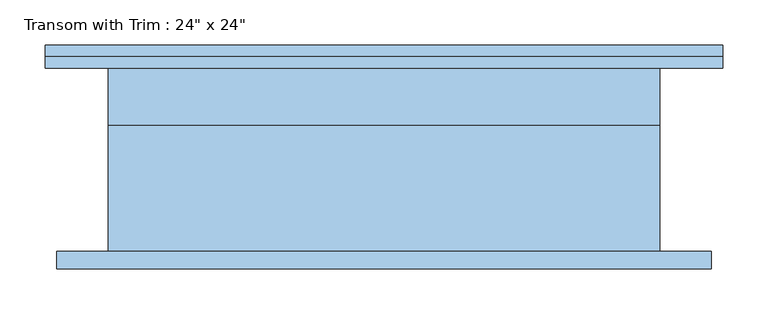
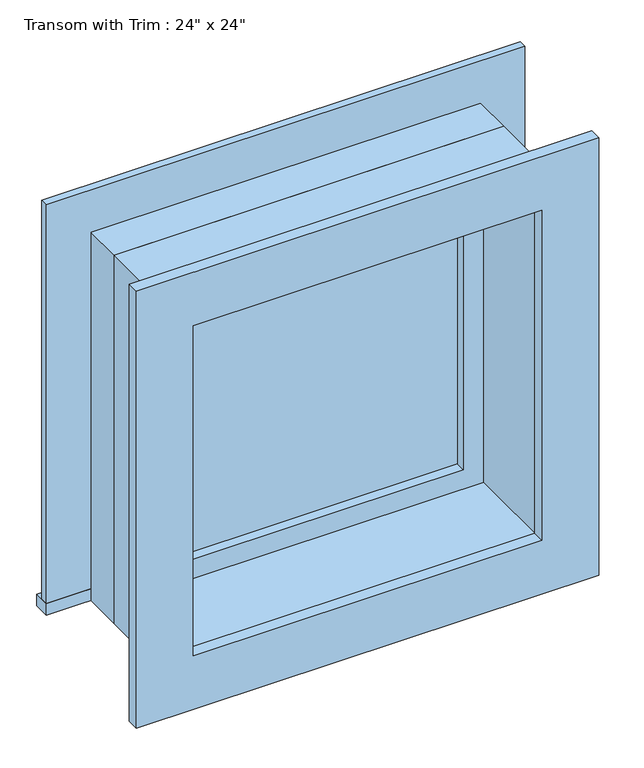
"""IFC4 building model written with IfcOpenShell, lengths in millimetres: window geometry."""

from ifc_helpers import new_model, si_unit, frame, origin, place, context, project, spatial, polyline, outline, extrude, source, transform, mapped, element, save


def window_e41d21a6(model_context):
    return source(origin(), model_context, "Body", "SweptSolid", [
        extrude(outline(polyline([(-412.75, 127.0), (336.55, 127.0), (336.55, 101.6), (-412.75, 101.6), (-412.75, 127.0)])), frame((0.0, 0.0, 2159.0), z_axis=(0.0, 0.0, 1.0), x_axis=(1.0, 0.0, 0.0)), (0.0, 0.0, 1.0), 19.05),
        extrude(outline(polyline([(2749.55, -323.85), (2749.55, 247.65), (2178.05, 247.65), (2178.05, 336.55), (2838.45, 336.55), (2838.45, -412.75), (2178.05, -412.75), (2178.05, -323.85), (2749.55, -323.85)])), frame((0.0, 101.6, 0.0), z_axis=(0.0, 1.0, 0.0), x_axis=(0.0, 0.0, 1.0)), (0.0, 0.0, 1.0), 12.7),
        extrude(outline(polyline([(2825.75, 323.85), (2825.75, -400.05), (2101.85, -400.05), (2101.85, 323.85), (2825.75, 323.85)]), holes=[polyline([(2736.85, 234.95), (2190.75, 234.95), (2190.75, -311.15), (2736.85, -311.15), (2736.85, 234.95)])]), frame((0.0, -120.65, 0.0), z_axis=(0.0, 1.0, 0.0), x_axis=(0.0, 0.0, 1.0)), (0.0, 0.0, 1.0), 19.05),
        extrude(outline(polyline([(203.2, 53.975), (-279.4, 53.975), (-279.4, 66.675), (203.2, 66.675), (203.2, 53.975)])), frame((0.0, 0.0, 2222.5), z_axis=(0.0, 0.0, 1.0), x_axis=(1.0, 0.0, 0.0)), (0.0, 0.0, 1.0), 482.6),
        extrude(outline(polyline([(2749.55, -323.85), (2178.05, -323.85), (2178.05, 247.65), (2749.55, 247.65), (2749.55, -323.85)]), holes=[polyline([(2705.1, -279.4), (2705.1, 203.2), (2222.5, 203.2), (2222.5, -279.4), (2705.1, -279.4)])]), frame((0.0, 38.1, 0.0), z_axis=(0.0, 1.0, 0.0), x_axis=(0.0, 0.0, 1.0)), (0.0, 0.0, 1.0), 44.45),
        extrude(outline(polyline([(2768.6, -342.9), (2159.0, -342.9), (2159.0, 266.7), (2768.6, 266.7), (2768.6, -342.9)]), holes=[polyline([(2736.85, -311.15), (2736.85, 234.95), (2190.75, 234.95), (2190.75, -311.15), (2736.85, -311.15)])]), frame((0.0, -101.6, 0.0), z_axis=(0.0, 1.0, 0.0), x_axis=(0.0, 0.0, 1.0)), (0.0, 0.0, 1.0), 139.7),
        extrude(outline(polyline([(2768.6, 266.7), (2768.6, -342.9), (2159.0, -342.9), (2159.0, 266.7), (2768.6, 266.7)]), holes=[polyline([(2749.55, 247.65), (2178.05, 247.65), (2178.05, -323.85), (2749.55, -323.85), (2749.55, 247.65)])]), frame((0.0, 38.1, 0.0), z_axis=(0.0, 1.0, 0.0), x_axis=(0.0, 0.0, 1.0)), (0.0, 0.0, 1.0), 63.5),
    ])


if __name__ == "__main__":
    model = new_model("IFC4")
    model_context = context("Model", 3, world=origin())
    ifc_project = project(units=[si_unit("LENGTHUNIT", "METRE", prefix="MILLI")], contexts=[model_context])
    site = spatial("IfcSite", under=ifc_project)
    building = spatial("IfcBuilding", under=site)
    placement = place(None, origin())
    window_shape = window_e41d21a6(model_context)
    element("IfcWindow", 1, ObjectType="Transom with Trim : 24\" x 24\"", at=placement, inside=building, context=model_context, shape_type="MappedRepresentation", body=[
        mapped(window_shape, transform((0.0, 0.0, 0.0), x_axis=(1.0, 0.0, 0.0), y_axis=(0.0, 1.0, 0.0), z_axis=(0.0, 0.0, 1.0))),
    ])
    save(model, "model.ifc")

# Revit data of these elements
# Type "Transom with Trim : 24\" x 24\""
#   Type Mark = "19"
#   Construction Type Id = "GSP4R"
#   Assembly Code = "B2020100"
#   Analytic Construction = "1/8 in Pilkington single glazing"
#   Visual Light Transmittance = 0.9
#   Solar Heat Gain Coefficient = 0.78
#   Heat Transfer Coefficient (U) = 0.6496 BTU/(h·ft²·°F)
#   Height = 2' - 0"
#   Default Sill Height = 7' - 1"
#   Trim Projection - Ext. = 0' - 0 1/2"
#   Trim Projection - Int. = 0' - 0 3/4"
#   Trim Width - Exterior = 0' - 3 1/2"
#   Trim Width - Interior = 0' - 3 1/2"
#   Width = 2' - 0"
#   Window Inset = 0' - 0 3/4"
#   Define Thermal Properties by = 1
#   Glass Pane Material = Glass
#   Sash Material = Sash
#   Trim Exterior Material = Trim
#   Trim Interior Material = Trim
#   Wall Closure = (empty or 0)
# Element 1 (IfcWindow, "Transom with Trim : 24\" x 24\"")
#   Materials on its faces: "Sash", "Trim", "Glass"
# Materials
#   "Glass": class "Glass", colour RGB 0 128 192, transparency 0.75, Description = "Soda Lime Glass", Cost = 0
#   "Sash": class "Wood", colour RGB 224 178 126, transparency 0
#   "Trim": class "Wood", colour RGB 224 178 126, transparency 0
